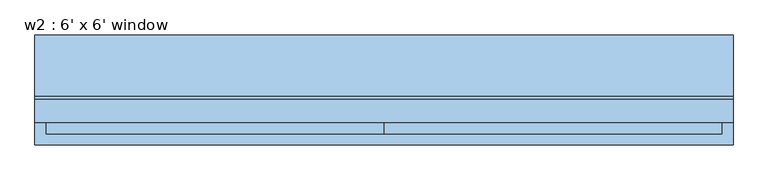
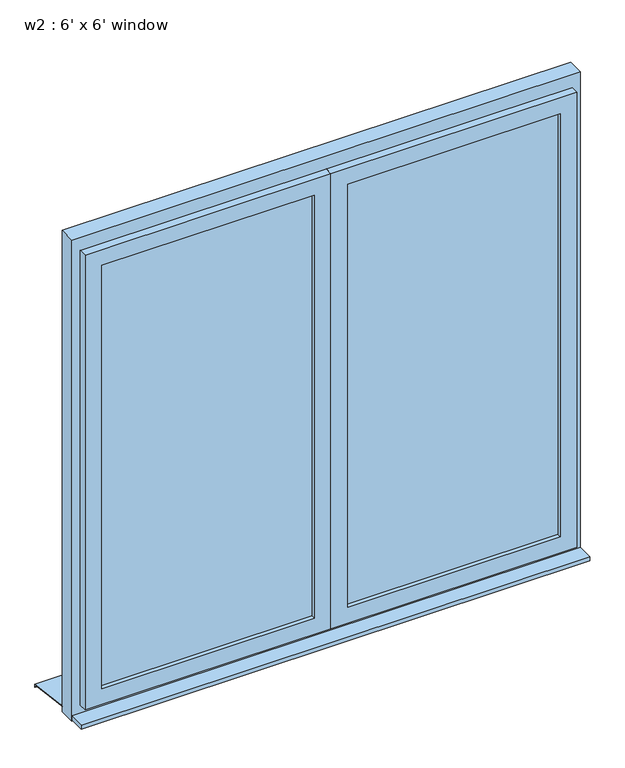
"""IFC4 building model written with IfcOpenShell, lengths in millimetres: window geometry, w2 : 6' x 6' window."""

from ifc_helpers import new_model, si_unit, frame, origin, place, context, project, spatial, polyline, outline, extrude, faceted_brep, source, transform, mapped, element, save


def w2_6_x_6_window_82e362f5(model_context):
    return source(origin(), model_context, "Body", "SolidModel", [
        extrude(outline(polyline([(-15.6778457, 1020.0), (144.3, 1000.0), (144.3, 990.0), (142.3, 990.0), (142.3, 998.3604634), (-15.8759277, 1018.0), (-25.7, 1018.0), (-25.7, 1020.0), (-15.6778457, 1020.0)])), frame((-914.4, 0.0, 0.0), z_axis=(1.0, 0.0, 0.0), x_axis=(0.0, 1.0, 0.0)), (0.0, 0.0, 1.0), 1828.8),
        extrude(outline(polyline([(-914.4, -144.3), (-914.4, -85.7), (914.4, -85.7), (914.4, -144.3), (-914.4, -144.3)])), frame((0.0, 0.0, 1005.0), z_axis=(0.0, 0.0, 1.0), x_axis=(1.0, 0.0, 0.0)), (0.0, 0.0, 1.0), 15.0),
        extrude(outline(polyline([(60.0, -70.7), (824.4, -70.7), (824.4, -100.7), (60.0, -100.7), (60.0, -70.7)])), frame((0.0, 0.0, 1110.0), z_axis=(0.0, 0.0, 1.0), x_axis=(1.0, 0.0, 0.0)), (0.0, 0.0, 1.0), 1608.8),
        extrude(outline(polyline([(-824.4, -70.7), (-60.0, -70.7), (-60.0, -100.7), (-824.4, -100.7), (-824.4, -70.7)])), frame((0.0, 0.0, 1110.0), z_axis=(0.0, 0.0, 1.0), x_axis=(1.0, 0.0, 0.0)), (0.0, 0.0, 1.0), 1608.8),
        extrude(outline(polyline([(2828.8, -914.4), (1000.0, -914.4), (1000.0, 914.4), (2828.8, 914.4), (2828.8, -914.4)]), holes=[polyline([(2748.8, -854.4), (2748.8, 854.4), (1080.0, 854.4), (1080.0, -854.4), (2748.8, -854.4)])]), frame((0.0, -85.7, 0.0), z_axis=(0.0, 1.0, 0.0), x_axis=(0.0, 0.0, 1.0)), (0.0, 0.0, 1.0), 60.0),
        extrude(outline(polyline([(30.0, -85.7), (-30.0, -85.7), (-30.0, -25.7), (30.0, -25.7), (30.0, -85.7)])), frame((0.0, 0.0, 1080.0), z_axis=(0.0, 0.0, 1.0), x_axis=(1.0, 0.0, 0.0)), (0.0, 0.0, 1.0), 1668.8),
        faceted_brep([(30.0, -85.7, 1080.0), (30.0, -55.7, 1080.0), (854.4, -55.7, 1080.0), (854.4, -85.7, 1080.0), (854.4, -55.7, 2748.8), (854.4, -85.7, 2748.8), (30.0, -55.7, 2748.8), (824.4, -55.7, 2718.8), (60.0, -55.7, 2718.8), (60.0, -55.7, 1110.0), (824.4, -55.7, 1110.0), (884.4, -85.7, 1050.0), (0.0, -85.7, 1050.0), (0.0, -85.7, 2778.8), (884.4, -85.7, 2778.8), (30.0, -85.7, 2748.8), (0.0, -115.7, 1050.0), (884.4, -115.7, 1050.0), (884.4, -115.7, 2778.8), (0.0, -115.7, 2778.8), (824.4, -115.7, 1110.0), (60.0, -115.7, 1110.0), (60.0, -115.7, 2718.8), (824.4, -115.7, 2718.8)], [[[0, 1, 2, 3]], [[3, 2, 4, 5]], [[2, 1, 6, 4], [7, 8, 9, 10]], [[11, 12, 13, 14], [5, 15, 0, 3]], [[16, 12, 11, 17]], [[17, 11, 14, 18]], [[18, 19, 16, 17], [20, 21, 22, 23]], [[9, 21, 20, 10]], [[10, 20, 23, 7]], [[15, 6, 1, 0]], [[19, 13, 12, 16]], [[8, 22, 21, 9]], [[5, 4, 6, 15]], [[18, 14, 13, 19]], [[7, 23, 22, 8]]]),
        faceted_brep([(-854.4, -85.7, 1080.0), (-854.4, -55.7, 1080.0), (-30.0, -55.7, 1080.0), (-30.0, -85.7, 1080.0), (-30.0, -55.7, 2748.8), (-30.0, -85.7, 2748.8), (-854.4, -55.7, 2748.8), (-60.0, -55.7, 2718.8), (-824.4, -55.7, 2718.8), (-824.4, -55.7, 1110.0), (-60.0, -55.7, 1110.0), (0.0, -85.7, 1050.0), (-884.4, -85.7, 1050.0), (-884.4, -85.7, 2778.8), (0.0, -85.7, 2778.8), (-854.4, -85.7, 2748.8), (-884.4, -115.7, 1050.0), (0.0, -115.7, 1050.0), (0.0, -115.7, 2778.8), (-884.4, -115.7, 2778.8), (-60.0, -115.7, 1110.0), (-824.4, -115.7, 1110.0), (-824.4, -115.7, 2718.8), (-60.0, -115.7, 2718.8)], [[[0, 1, 2, 3]], [[3, 2, 4, 5]], [[2, 1, 6, 4], [7, 8, 9, 10]], [[11, 12, 13, 14], [5, 15, 0, 3]], [[16, 12, 11, 17]], [[17, 11, 14, 18]], [[18, 19, 16, 17], [20, 21, 22, 23]], [[9, 21, 20, 10]], [[10, 20, 23, 7]], [[15, 6, 1, 0]], [[19, 13, 12, 16]], [[8, 22, 21, 9]], [[5, 4, 6, 15]], [[18, 14, 13, 19]], [[7, 23, 22, 8]]]),
    ])


if __name__ == "__main__":
    model = new_model("IFC4")
    model_context = context("Model", 3, world=origin())
    ifc_project = project(units=[si_unit("LENGTHUNIT", "METRE", prefix="MILLI")], contexts=[model_context])
    site = spatial("IfcSite", under=ifc_project)
    building = spatial("IfcBuilding", under=site)
    placement = place(None, origin())
    w2_6_x_6_window_shape = w2_6_x_6_window_82e362f5(model_context)
    element("IfcWindow", 1, ObjectType="w2 : 6' x 6' window", at=placement, inside=building, context=model_context, shape_type="MappedRepresentation", body=[
        mapped(w2_6_x_6_window_shape, transform((0.0, 0.0, 0.0), x_axis=(1.0, 0.0, 0.0), y_axis=(0.0, 1.0, 0.0), z_axis=(0.0, 0.0, 1.0))),
    ])
    save(model, "model.ifc")

# Revit data of these elements
# Type "w2 : 6' x 6' window"
#   Type Mark = "27"
#   Operation = "DoublePanelVertical"
#   Keynote = "16.05.01"
#   Analytic Construction = "<None>"
#   Rough Width = 6' - 0"
#   Rough Height = 6' - 0"
#   Rahmentiefe = 0' - 2.3622"
#   Rahmenhöhe unten = 0' - 3.14961"
#   Rahmehöhe oben = 0' - 3.14961"
#   Rahmenbreite = 0' - 2.3622"
#   Heat Transfer Coefficient (U) = 2.81836 BTU/(h·ft²·°F)
#   Height = 6' - 0"
#   Flügeltiefe = 0' - 2.3622"
#   Flügelbreite = 0' - 2.3622"
#   Einbautiefe (von außen) [instance default] = 0' - 5.51181"
#   Width = 6' - 0"
#   Kippflügel [instance default] = yes
#   Drehflügel im Grundriß darstellen [instance default] = no
#   Drehflügel [instance default] = yes
#   Define Thermal Properties by = 1
#   Rahmen [instance default] = none
#   Glas [instance default] = blue glass
#   Flügel [instance default] = WINDOW COLOUR WHITE
#   Fensterbank aussen [instance default] = WINDOW COLOUR WHITE
#   Fensterbank innen [instance default] = WINDOW COLOUR WHITE
#   Visual Light Transmittance = 0
#   Thermal Resistance (R) = 0
#   Solar Heat Gain Coefficient = 0
#   Wall Closure = (empty or 0)
# Element 1 (IfcWindow, "w2 : 6' x 6' window")
#   Materials on its faces: "WINDOW COLOUR WHITE", "blue glass"
# Materials
#   "blue glass": class "System", colour RGB 0 0 255, transparency 0.75, Cost = 0
#   "WINDOW COLOUR WHITE": class "Generic", colour RGB 120 120 120, transparency 0, Cost = 0
